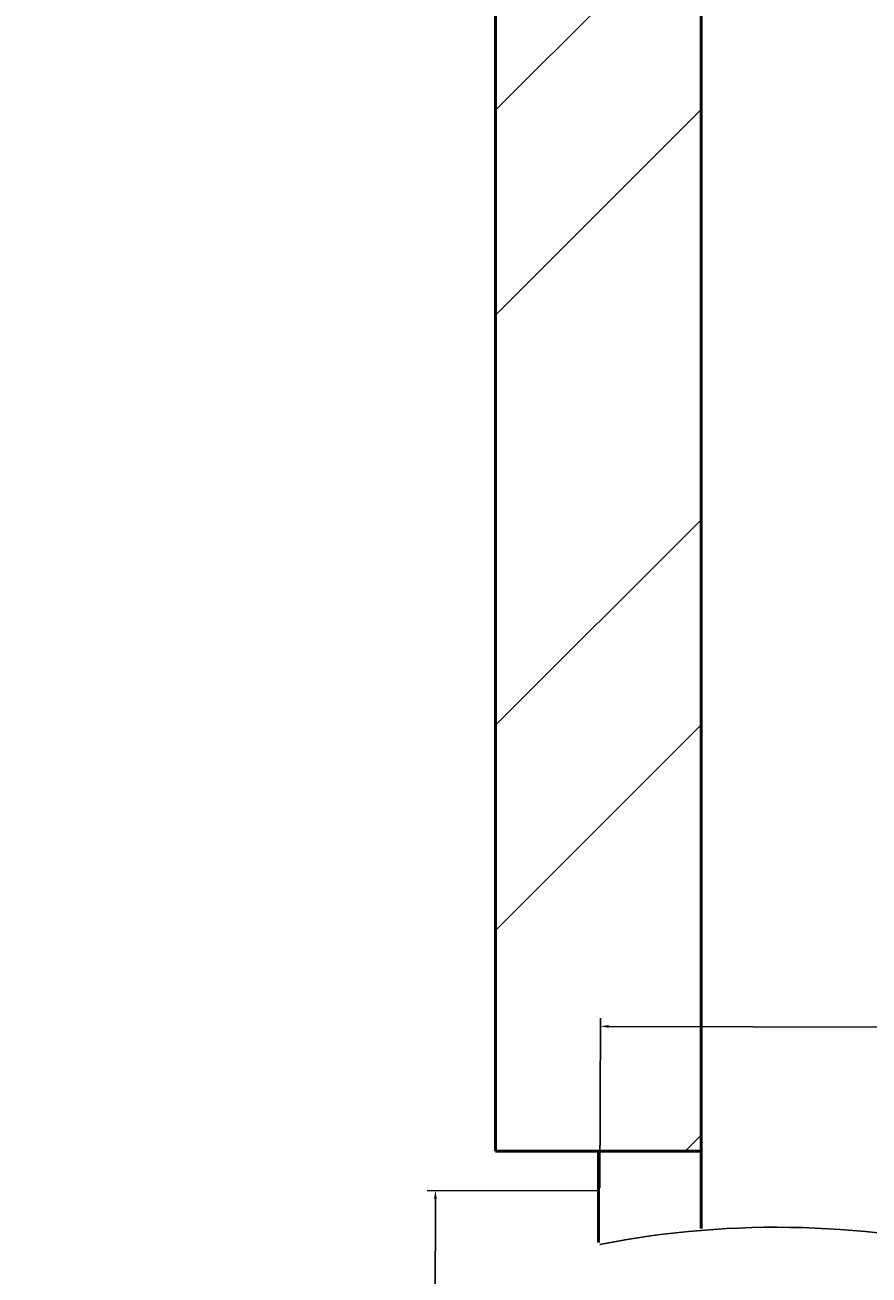
# Model space of a CAD drawing. Units: inches. Extents: x 1901 to 2863, y 888 to 2433.
# Tile 82 of 91: x 2645 to 2663, y 2037 to 2064. Entities that reach past the tile are written whole.
import ezdxf

# ---------------------------------------------------------------- set-up
doc = ezdxf.new("R2010")
doc.units = ezdxf.units.IN
for name, color, linetype, lineweight in [('A-ANNO-DIMS', 2, 'Continuous', 18), ('A-DOOR', 4, 'Continuous', 25), ('A-WALL', 7, 'Continuous', 50), ('A-WALL-PATT', 8, 'Continuous', 13)]:
    doc.layers.add(name, color=color, linetype=linetype, lineweight=lineweight)
doc.styles.get("Standard").update_dxf_attribs({"font": 'arial.ttf'})
doc.dimstyles.get("Standard").update_dxf_attribs({"dimtxt": 0.18, "dimasz": 0.18, "dimexe": 0.18, "dimexo": 0.0625, "dimgap": 0.09, "dimtad": 0, "dimtih": 1, "dimtoh": 1, "dimdec": 4, "dimzin": 0, "dimdsep": 46, "dimtxsty": 'Standard', "dimcen": 0.09, "dimadec": 0, "dimazin": 0, "dimtfac": 1, "dimtdec": 4, "dimtofl": 0, "dimtmove": 0, "dimatfit": 3, "dimfxl": 1, "dimtolj": 1, "dimtzin": 0, "dimarcsym": 0})

# ---------------------------------------------------------------- blocks, each defined once
blk = doc.blocks.new('DOOR-20B')
blk.add_line((0.002, -0.016), (0.002, 23.984))
blk.add_arc((0.002, 3.902), 20.082, 348.7487, 90)
blk = doc.blocks.new('*D39')
at = {"layer": 'A-ANNO-DIMS', "color": 0, "lineweight": -2, "transparency": 16777216}
for p, q in [((2657.208, 2038.63), (2657.218, 2042.347)), ((2657.397, 2042.167), (2668.086, 2042.138)), ((2681.037, 2042.102), (2670.349, 2042.131)), ((2681.208, 2038.564), (2681.218, 2042.282))]:
    blk.add_line(p, q, dxfattribs=at)
at = {"layer": 'A-ANNO-DIMS', "color": 0, "transparency": 16777216}
for points in [[(2657.397, 2042.197), (2657.397, 2042.137), (2657.217, 2042.167)], [(2681.037, 2042.132), (2681.037, 2042.072), (2681.217, 2042.102)]]:
    blk.add_solid(points, dxfattribs=at)
at = {"layer": 'Defpoints', "color": 0, "transparency": 16777216}
for p in [(2681.217, 2042.102), (2657.208, 2038.567), (2681.207, 2038.502)]:
    blk.add_point(p, dxfattribs=at)
at = {"layer": 'A-ANNO-DIMS', "color": 0, "transparency": 16777216, "insert": (2669.217, 2042.134), "char_height": 0.18, "attachment_point": 5}
blk.add_mtext('\\A1;DOOR D5 24 TYP.', dxfattribs=at)
blk = doc.blocks.new('*D40')
at = {"layer": 'A-ANNO-DIMS', "color": 0, "lineweight": -2, "transparency": 16777216}
for p, q in [((2657.145, 2038.567), (2653.428, 2038.577)), ((2653.607, 2038.397), (2653.58, 2028.323)), ((2653.551, 2017.888), (2653.579, 2027.962)), ((2657.088, 2017.698), (2653.371, 2017.708))]:
    blk.add_line(p, q, dxfattribs=at)
at = {"layer": 'A-ANNO-DIMS', "color": 0, "transparency": 16777216}
for points in [[(2653.577, 2038.397), (2653.637, 2038.397), (2653.608, 2038.577)], [(2653.521, 2017.888), (2653.581, 2017.888), (2653.551, 2017.708)]]:
    blk.add_solid(points, dxfattribs=at)
at = {"layer": 'Defpoints', "color": 0, "transparency": 16777216}
for p in [(2653.608, 2038.577), (2657.208, 2038.567), (2657.151, 2017.698)]:
    blk.add_point(p, dxfattribs=at)
at = {"layer": 'A-ANNO-DIMS', "color": 0, "transparency": 16777216, "insert": (2653.579, 2028.142), "char_height": 0.18, "attachment_point": 5}
blk.add_mtext('\\A1;21 TYP.', dxfattribs=at)

msp = doc.modelspace()

# ---------------------------------------------------------------- hatches: boundary and pattern name
at = {"layer": 'A-WALL-PATT'}
h = msp.add_hatch(dxfattribs=at)
h.set_pattern_fill('ANSI32', color=256)
h.paths.add_polyline_path([(2192.501, 2274.134), (2141.264, 2274.134), (2141.264, 2269.634), (2192.501, 2269.634)])
h.paths.add_polyline_path([(2259.926, 2274.134), (2216.501, 2274.134), (2216.501, 2269.634), (2255.426, 2269.634), (2255.426, 2214.634), (2250.809, 2214.634), (2250.809, 2210.134), (2259.926, 2210.134), (2259.926, 2215.134), (2271.756, 2215.134), (2271.756, 2217.384), (2271.756, 2219.634), (2259.926, 2219.634)])
h.paths.add_polyline_path([(2171.426, 2269.634), (2166.926, 2269.634), (2166.926, 2219.634), (2121.238, 2219.634), (2121.238, 2215.134), (2166.926, 2215.134), (2166.926, 2083.134), (2161.807, 2083.134), (2161.807, 2078.634), (2171.426, 2078.634), (2176.996, 2078.634), (2176.996, 2080.884), (2176.996, 2083.134), (2171.426, 2083.134), (2171.426, 2210.134), (2230.912, 2210.134), (2230.912, 2212.384), (2230.912, 2214.634), (2171.426, 2214.634)])
h.paths.add_polyline_path([(2117.264, 2274.134), (2089.426, 2274.134), (2089.426, 2219.634), (2081.136, 2219.634), (2081.136, 2215.134), (2089.426, 2215.134), (2098.004, 2215.134), (2098.004, 2217.384), (2098.004, 2219.634), (2093.926, 2219.634), (2093.926, 2269.634), (2117.264, 2269.634), (2117.264, 2271.884)])
h.paths.add_polyline_path([(2343.426, 2219.634), (2329.295, 2219.634), (2329.295, 2215.134), (2338.926, 2215.134), (2338.926, 2184.739), (2343.426, 2184.739)])
h.paths.add_polyline_path([(2338.926, 2083.134), (2329.295, 2083.134), (2208.966, 2083.134), (2208.966, 2078.634), (2338.926, 2078.634)])
h.paths.add_polyline_path([(2343.426, 2136.739), (2338.926, 2136.739), (2338.926, 1872.634), (2343.426, 1872.634)])
h.paths.add_polyline_path([(2343.426, 1863.634), (2397.68, 1863.634), (2397.68, 1821.634), (2384.138, 1821.634), (2384.138, 1812.634), (2418.33, 1812.634), (2418.33, 1817.134), (2418.33, 1821.634), (2406.68, 1821.634), (2406.68, 1863.634), (2459.499, 1863.634), (2459.499, 1821.634), (2447.138, 1821.634), (2447.138, 1812.634), (2459.499, 1812.634), (2468.499, 1812.634), (2468.499, 1872.634), (2394.426, 1872.634), (2334.426, 1872.634), (2334.426, 1812.634), (2343.426, 1812.634), (2353.251, 1812.634), (2353.251, 1821.634), (2343.426, 1821.634)])
h.paths.add_polyline_path([(2510.014, 1872.634), (2468.499, 1872.634), (2468.499, 1868.134), (2510.014, 1868.134)])
h.paths.add_polyline_path([(2514.009, 1817.134), (2468.499, 1817.134), (2468.499, 1812.634), (2482.114, 1812.634), (2482.114, 1800.606), (2486.614, 1800.606), (2486.614, 1812.634), (2514.009, 1812.634)])
h.paths.add_polyline_path([(2299.247, 1814.884), (2299.247, 1817.134), (2295.926, 1817.134), (2295.926, 1854.169), (2293.676, 1854.169), (2291.426, 1854.169), (2291.426, 1817.134), (2266.109, 1817.134), (2266.109, 1812.634), (2299.247, 1812.634)])
h.paths.add_polyline_path([(2218.109, 1817.134), (2206.46, 1817.134), (2171.426, 1817.134), (2171.426, 1949.134), (2190.1, 1949.134), (2190.1, 1953.634), (2163.468, 1953.634), (2163.468, 1949.134), (2166.926, 1949.134), (2166.926, 1817.134), (2114.297, 1817.134), (2114.297, 1812.634), (2218.109, 1812.634)])
h.paths.add_polyline_path([(2029.426, 1970.922), (2024.926, 1970.922), (2024.926, 1912.717), (2029.426, 1912.717)])
h.paths.add_polyline_path([(2132.297, 1953.634), (2113.926, 1953.634), (2113.926, 1975.888), (2111.676, 1975.888), (2109.426, 1975.888), (2109.426, 1953.634), (2029.426, 1953.634), (2029.426, 1949.134), (2132.297, 1949.134)])
h.paths.add_polyline_path([(2029.426, 1853.606), (2029.31, 1853.606), (2029.31, 1853.606), (2029.426, 1853.606), (2029.426, 1864.717), (2024.926, 1864.717), (2024.926, 1812.634), (2066.297, 1812.634), (2066.297, 1814.884), (2066.297, 1817.134), (2029.426, 1817.134)])
h.paths.add_polyline_path([(2122.926, 2010.088), (2120.676, 2010.088), (2118.426, 2010.088), (2118.426, 2006.134), (2029.426, 2006.134), (2029.426, 2001.634), (2109.426, 2001.634), (2109.426, 1998.041), (2113.926, 1998.041), (2113.926, 2001.634), (2122.926, 2001.634)])
h.paths.add_polyline_path([(2029.426, 2031.376), (2024.926, 2031.376), (2024.926, 1994.922), (2027.176, 1994.922), (2029.426, 1994.922)])
h.paths.add_polyline_path([(2029.426, 2136.739), (2024.926, 2136.739), (2024.926, 2067.376), (2027.176, 2067.376), (2029.426, 2067.376)])
h.paths.add_polyline_path([(2125.618, 2083.134), (2029.426, 2083.134), (2029.426, 2078.634), (2118.426, 2078.634), (2118.426, 2030.715), (2122.926, 2030.715), (2122.926, 2078.634), (2125.618, 2078.634)])
h.paths.add_polyline_path([(2029.426, 2215.134), (2040.468, 2215.134), (2040.468, 2217.384), (2040.468, 2219.634), (2024.926, 2219.634), (2024.926, 2184.739), (2029.426, 2184.739), (2029.426, 2187.778)])
h.paths.add_polyline_path([(2686.426, 2274.134), (2659.284, 2274.134), (2659.284, 2269.634), (2681.926, 2269.634), (2681.926, 2219.634), (2676.816, 2219.634), (2676.816, 2215.134), (2681.926, 2215.134), (2697.011, 2215.134), (2697.011, 2217.384), (2697.011, 2219.634), (2686.426, 2219.634)])
h.paths.add_polyline_path([(2609.926, 2269.634), (2635.284, 2269.634), (2635.284, 2274.134), (2571.431, 2274.134), (2571.431, 2269.634), (2605.426, 2269.634), (2605.426, 2214.634), (2549.098, 2214.634), (2549.098, 2210.134), (2605.426, 2210.134), (2605.426, 2083.134), (2601.014, 2083.134), (2601.014, 2080.884), (2601.014, 2078.634), (2609.926, 2078.634), (2616.162, 2078.634), (2616.162, 2080.884), (2616.162, 2083.134), (2609.926, 2083.134), (2609.926, 2215.134), (2651.465, 2215.134), (2651.465, 2217.384), (2651.465, 2219.634), (2609.926, 2219.634)])
h.paths.add_polyline_path([(2521.426, 2269.634), (2547.431, 2269.634), (2547.431, 2271.884), (2547.431, 2274.134), (2516.926, 2274.134), (2516.926, 2219.634), (2506.41, 2219.634), (2506.41, 2215.134), (2516.926, 2215.134), (2516.926, 2210.134), (2525.402, 2210.134), (2525.402, 2212.384), (2525.402, 2214.634), (2521.426, 2214.634)])
h.paths.add_polyline_path([(2456.011, 2219.634), (2439.426, 2219.634), (2439.426, 2187.888), (2443.926, 2187.888), (2443.926, 2215.134), (2456.011, 2215.134)])
h.paths.add_polyline_path([(2752.926, 2219.634), (2739.485, 2219.634), (2739.485, 2215.134), (2748.426, 2215.134), (2748.426, 2187.888), (2752.926, 2187.888)])
h.paths.add_polyline_path([(2752.926, 2139.888), (2748.426, 2139.888), (2748.426, 2083.134), (2648.416, 2083.134), (2648.416, 2078.634), (2654.926, 2078.634), (2654.926, 2039.437), (2659.426, 2039.437), (2659.426, 2078.634), (2748.426, 2078.634), (2748.426, 2063.429), (2752.926, 2063.429)])
h.paths.add_polyline_path([(2752.926, 2010.634), (2659.426, 2010.634), (2659.426, 2015.652), (2654.926, 2015.652), (2654.926, 2010.634), (2605.426, 2010.634), (2605.426, 1920.967), (2609.926, 1920.967), (2609.926, 2006.134), (2748.426, 2006.134), (2748.426, 1982.466), (2752.926, 1982.466)])
h.paths.add_polyline_path([(2752.926, 2027.429), (2748.426, 2027.429), (2748.426, 2010.634), (2752.926, 2010.634)])
h.paths.add_polyline_path([(2748.426, 1886.134), (2609.926, 1886.134), (2609.926, 1889.719), (2605.426, 1889.719), (2605.426, 1861.262), (2609.926, 1861.262), (2609.926, 1881.634), (2748.426, 1881.634)])
h.paths.add_polyline_path([(2456.855, 2228.831), (2498.401, 2228.831), (2498.401, 2247.488), (2456.855, 2247.488)], flags=9)
h.paths.add_polyline_path([(2038.602, 2237.418), (2080.174, 2237.418), (2080.174, 2256.075), (2038.602, 2256.075)], flags=9)
h.paths.add_polyline_path([(2292.009, 1062.394), (2539.932, 1062.394), (2539.932, 1099.487), (2292.009, 1099.487)], flags=9)
h.paths.add_polyline_path([(2424.91, 1832.253), (2448.513, 1832.253), (2448.513, 1846.678), (2424.91, 1846.678)], flags=25)
h.paths.add_polyline_path([(2359.076, 1832.253), (2382.678, 1832.253), (2382.678, 1846.678), (2359.076, 1846.678)], flags=25)
h.paths.add_polyline_path([(2352.899, 1684.802), (2367.543, 1684.802), (2367.543, 1697.167), (2352.899, 1697.167)], flags=9)
h.paths.add_polyline_path([(2079.288, 1755.826), (2169.024, 1755.826), (2169.024, 1774.372), (2079.288, 1774.372)], flags=9)
h.paths.add_polyline_path([(2404.09, 1373.857), (2404.09, 1463.593), (2385.544, 1463.593), (2385.544, 1373.857)], flags=9)
h.paths.add_polyline_path([(2268.091, 2236.371), (2309.636, 2236.371), (2309.636, 2255.028), (2268.091, 2255.028)], flags=9)
h.paths.add_polyline_path([(2575.96, 1700.951), (2665.696, 1700.951), (2665.696, 1719.498), (2575.96, 1719.498)], flags=9)
h.paths.add_polyline_path([(2302.962, 1878.474), (2329.524, 1878.474), (2329.524, 1888.777), (2302.962, 1888.777)], flags=9)
h.paths.add_polyline_path([(2097.415, 2240.576), (2126.573, 2240.576), (2126.573, 2259.233), (2097.415, 2259.233)], flags=9)
h.paths.add_polyline_path([(2208.725, 2246.124), (2237.882, 2246.124), (2237.882, 2264.781), (2208.725, 2264.781)], flags=9)
h.paths.add_polyline_path([(2038.147, 1925.958), (2076.987, 1925.958), (2076.987, 1944.615), (2038.147, 1944.615)], flags=9)
h.paths.add_polyline_path([(2239.144, 1926.672), (2288.465, 1926.672), (2288.465, 1945.329), (2239.144, 1945.329)], flags=9)
h.paths.add_polyline_path([(2175.429, 2007.33), (2212.356, 2007.33), (2212.356, 2025.987), (2175.429, 2025.987)], flags=9)
h.paths.add_polyline_path([(2225.034, 2091.794), (2263.875, 2091.794), (2263.875, 2110.451), (2225.034, 2110.451)], flags=9)
h.paths.add_polyline_path([(2035.398, 2098.478), (2074.238, 2098.478), (2074.238, 2117.135), (2035.398, 2117.135)], flags=9)
h.paths.add_polyline_path([(2050.102, 2029.209), (2083.26, 2029.209), (2083.26, 2047.866), (2050.102, 2047.866)], flags=9)
h.paths.add_polyline_path([(2069.677, 1956.719), (2098.835, 1956.719), (2098.835, 1975.376), (2069.677, 1975.376)], flags=25)
h.paths.add_polyline_path([(2328.62, 1753.336), (2361.663, 1753.336), (2361.663, 1771.993), (2328.62, 1771.993)], flags=9)
h.paths.add_polyline_path([(2395.162, 2060.888), (2395.162, 2140.654), (2378.676, 2140.654), (2378.676, 2060.888)], flags=9)
h.paths.add_polyline_path([(2463.728, 2059.02), (2492.886, 2059.02), (2492.886, 2077.677), (2463.728, 2077.677)], flags=9)
h.paths.add_polyline_path([(2458.027, 2181.536), (2496.868, 2181.536), (2496.868, 2200.194), (2458.027, 2200.194)], flags=9)
h.paths.add_polyline_path([(2527.577, 2243.074), (2556.735, 2243.074), (2556.735, 2261.731), (2527.577, 2261.731)], flags=9)
h.paths.add_polyline_path([(2694.461, 2232.767), (2736.033, 2232.767), (2736.033, 2251.425), (2694.461, 2251.425)], flags=9)
h.paths.add_polyline_path([(2637.821, 2249.225), (2666.979, 2249.225), (2666.979, 2267.882), (2637.821, 2267.882)], flags=9)
h.paths.add_polyline_path([(2623.687, 2183.541), (2662.528, 2183.541), (2662.528, 2202.199), (2623.687, 2202.199)], flags=9)
h.paths.add_polyline_path([(2691.965, 2021.5), (2725.124, 2021.5), (2725.124, 2040.157), (2691.965, 2040.157)], flags=9)
h.paths.add_polyline_path([(2621.043, 1975.912), (2662.335, 1975.912), (2662.335, 1994.569), (2621.043, 1994.569)], flags=25)
h.paths.add_polyline_path([(2479.032, 1927.62), (2519.844, 1927.62), (2519.844, 1946.277), (2479.032, 1946.277)], flags=9)
h.paths.add_polyline_path([(2670.941, 1849.076), (2716.005, 1849.076), (2716.005, 1867.734), (2670.941, 1867.734)], flags=9)
h.paths.add_polyline_path([(2523.613, 1782.956), (2550.175, 1782.956), (2550.175, 1793.26), (2523.613, 1793.26)], flags=9)
h.paths.add_polyline_path([(2450.841, 1207.331), (2492.386, 1207.331), (2492.386, 1225.989), (2450.841, 1225.989)], flags=9)
h.paths.add_polyline_path([(2527.751, 1203.841), (2556.908, 1203.841), (2556.908, 1222.499), (2527.751, 1222.499)], flags=9)
h.paths.add_polyline_path([(2639.111, 1207.2), (2668.268, 1207.2), (2668.268, 1225.857), (2639.111, 1225.857)], flags=9)
h.paths.add_polyline_path([(2692.594, 1218.965), (2734.167, 1218.965), (2734.167, 1237.623), (2692.594, 1237.623)], flags=9)
h.paths.add_polyline_path([(2669.266, 1366.329), (2708.106, 1366.329), (2708.106, 1384.987), (2669.266, 1384.987)], flags=9)
h.paths.add_polyline_path([(2463.313, 1358.031), (2502.153, 1358.031), (2502.153, 1376.688), (2463.313, 1376.688)], flags=9)
h.paths.add_polyline_path([(2494.725, 1449.963), (2531.652, 1449.963), (2531.652, 1468.62), (2494.725, 1468.62)], flags=9)
h.paths.add_polyline_path([(2675.565, 1422.157), (2708.724, 1422.157), (2708.724, 1440.815), (2675.565, 1440.815)], flags=9)
h.paths.add_polyline_path([(2685.634, 1493.891), (2714.792, 1493.891), (2714.792, 1512.548), (2685.634, 1512.548)], flags=9)
h.paths.add_polyline_path([(2686.805, 1529.913), (2725.645, 1529.913), (2725.645, 1548.57), (2686.805, 1548.57)], flags=9)
h.paths.add_polyline_path([(2503.651, 1537.991), (2552.972, 1537.991), (2552.972, 1556.648), (2503.651, 1556.648)], flags=9)
h.paths.add_polyline_path([(2291.713, 1643.504), (2318.275, 1643.504), (2318.275, 1653.807), (2291.713, 1653.807)], flags=9)
h.paths.add_polyline_path([(2450.626, 1610.52), (2477.189, 1610.52), (2477.189, 1620.824), (2450.626, 1620.824)], flags=9)
h.paths.add_polyline_path([(2359.985, 1551.814), (2422.253, 1551.814), (2422.253, 1562.117), (2359.985, 1562.117)], flags=9)
h.paths.add_polyline_path([(2280.106, 1249.006), (2321.651, 1249.006), (2321.651, 1267.663), (2280.106, 1267.663)], flags=9)
h.paths.add_polyline_path([(2164.057, 1274.232), (2193.215, 1274.232), (2193.215, 1292.889), (2164.057, 1292.889)], flags=9)
h.paths.add_polyline_path([(2118.21, 1277.694), (2151.252, 1277.694), (2151.252, 1296.351), (2118.21, 1296.351)], flags=9)
h.paths.add_polyline_path([(2031.946, 1268.529), (2073.519, 1268.529), (2073.519, 1287.187), (2031.946, 1287.187)], flags=9)
h.paths.add_polyline_path([(2050.199, 1409.079), (2089.04, 1409.079), (2089.04, 1427.736), (2050.199, 1427.736)], flags=9)
h.paths.add_polyline_path([(2243.743, 1421.032), (2282.584, 1421.032), (2282.584, 1439.689), (2243.743, 1439.689)], flags=9)
h.paths.add_polyline_path([(2190.746, 1509.769), (2231.558, 1509.769), (2231.558, 1528.426), (2190.746, 1528.426)], flags=9)
h.paths.add_polyline_path([(2058.392, 1475.415), (2091.55, 1475.415), (2091.55, 1494.073), (2058.392, 1494.073)], flags=9)
h.paths.add_polyline_path([(2062.447, 1553.09), (2091.605, 1553.09), (2091.605, 1571.747), (2062.447, 1571.747)], flags=9)
h.paths.add_polyline_path([(2219.524, 1590.365), (2266.147, 1590.365), (2266.147, 1609.022), (2219.524, 1609.022)], flags=9)
h.paths.add_polyline_path([(2041.072, 1584.188), (2079.912, 1584.188), (2079.912, 1602.845), (2041.072, 1602.845)], flags=9)

# ---------------------------------------------------------------- linework, layer by layer
at = {"layer": 'A-WALL'}
for p, q in [((2654.926, 2078.634), (2654.926, 2039.437)), ((2659.426, 2037.744), (2659.426, 2078.634)), ((2654.926, 2039.437), (2659.426, 2039.437)), ((2659.426, 2039.437), (2657.176, 2039.437)), ((2657.176, 2039.437), (2657.176, 2037.437))]:
    msp.add_line(p, q, dxfattribs=at)

# ---------------------------------------------------------------- block references
at = {"layer": 'A-DOOR', "extrusion": (0, 0, -1), "zscale": -1, "rotation": 90.1553947244059}
msp.add_blockref('DOOR-20B', (-2657.167, 2017.696), dxfattribs=at)

# ---------------------------------------------------------------- dimensions: what is measured, and where the dimension line sits
at = {"layer": 'A-ANNO-DIMS'}
for base, p1, p2, angle, text, picture, middle in [((2681.217, 2042.102), (2657.208, 2038.567), (2681.207, 2038.502), 359.8446, 'DOOR D5 <> TYP.', '*D39', (2669.217, 2042.134)), ((2653.608, 2038.577), (2657.151, 2017.698), (2657.208, 2038.567), 89.8446, '<> TYP.', '*D40', (2653.579, 2028.142))]:
    dim = msp.add_linear_dim(base=base, p1=p1, p2=p2, angle=angle, text=text, dimstyle='Standard', override={"dimdec": 0, "dimlfac": 1, "dimrnd": 0, "dimzin": 0, "dimdsep": 46, "dimlunit": 2}, dxfattribs=at)
    dim.commit()
    dim.dimension.update_dxf_attribs({"geometry": picture, "text_midpoint": middle})

doc.saveas('drawing.dxf')
